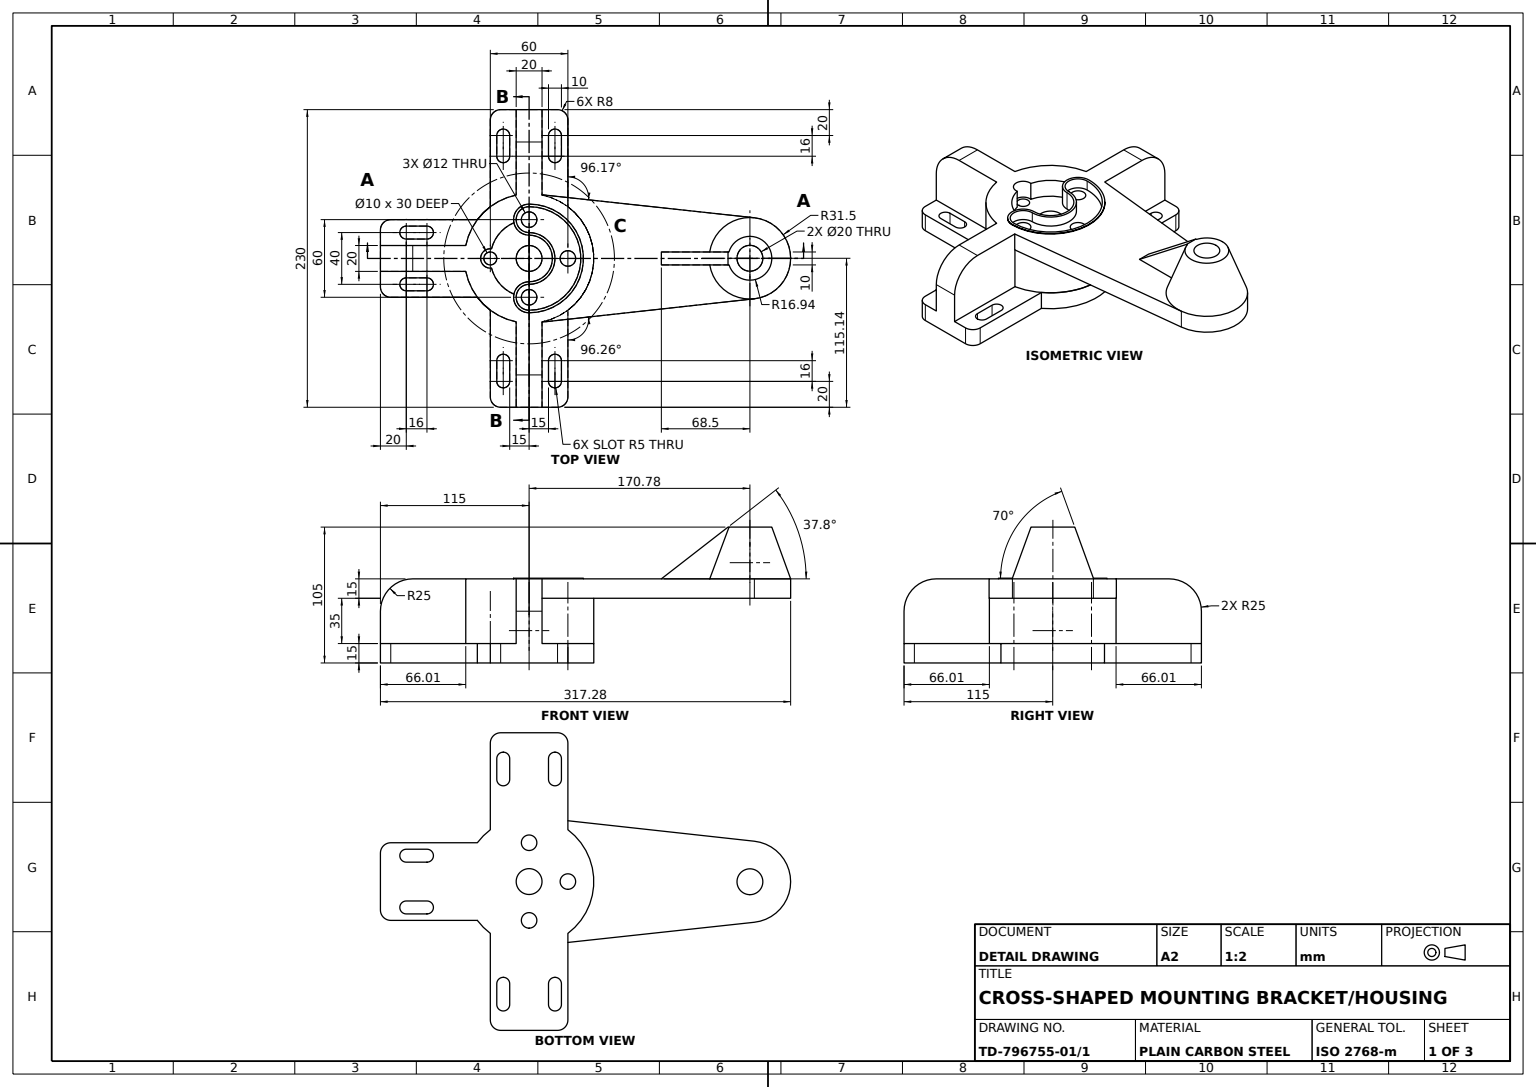
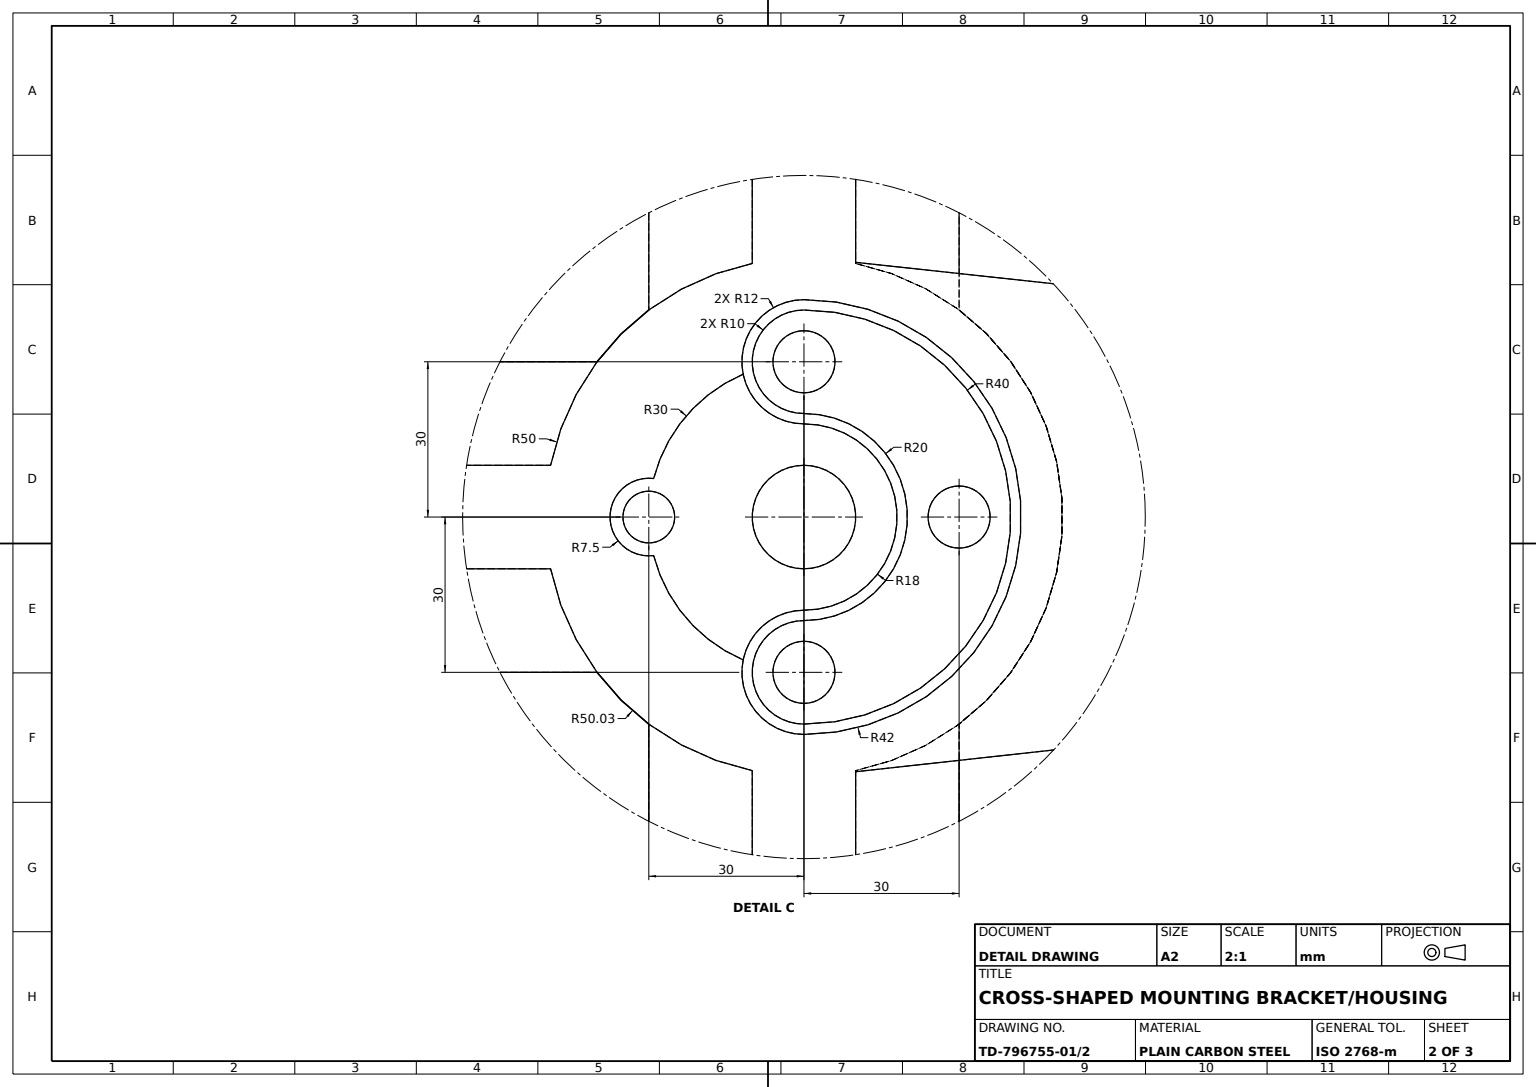
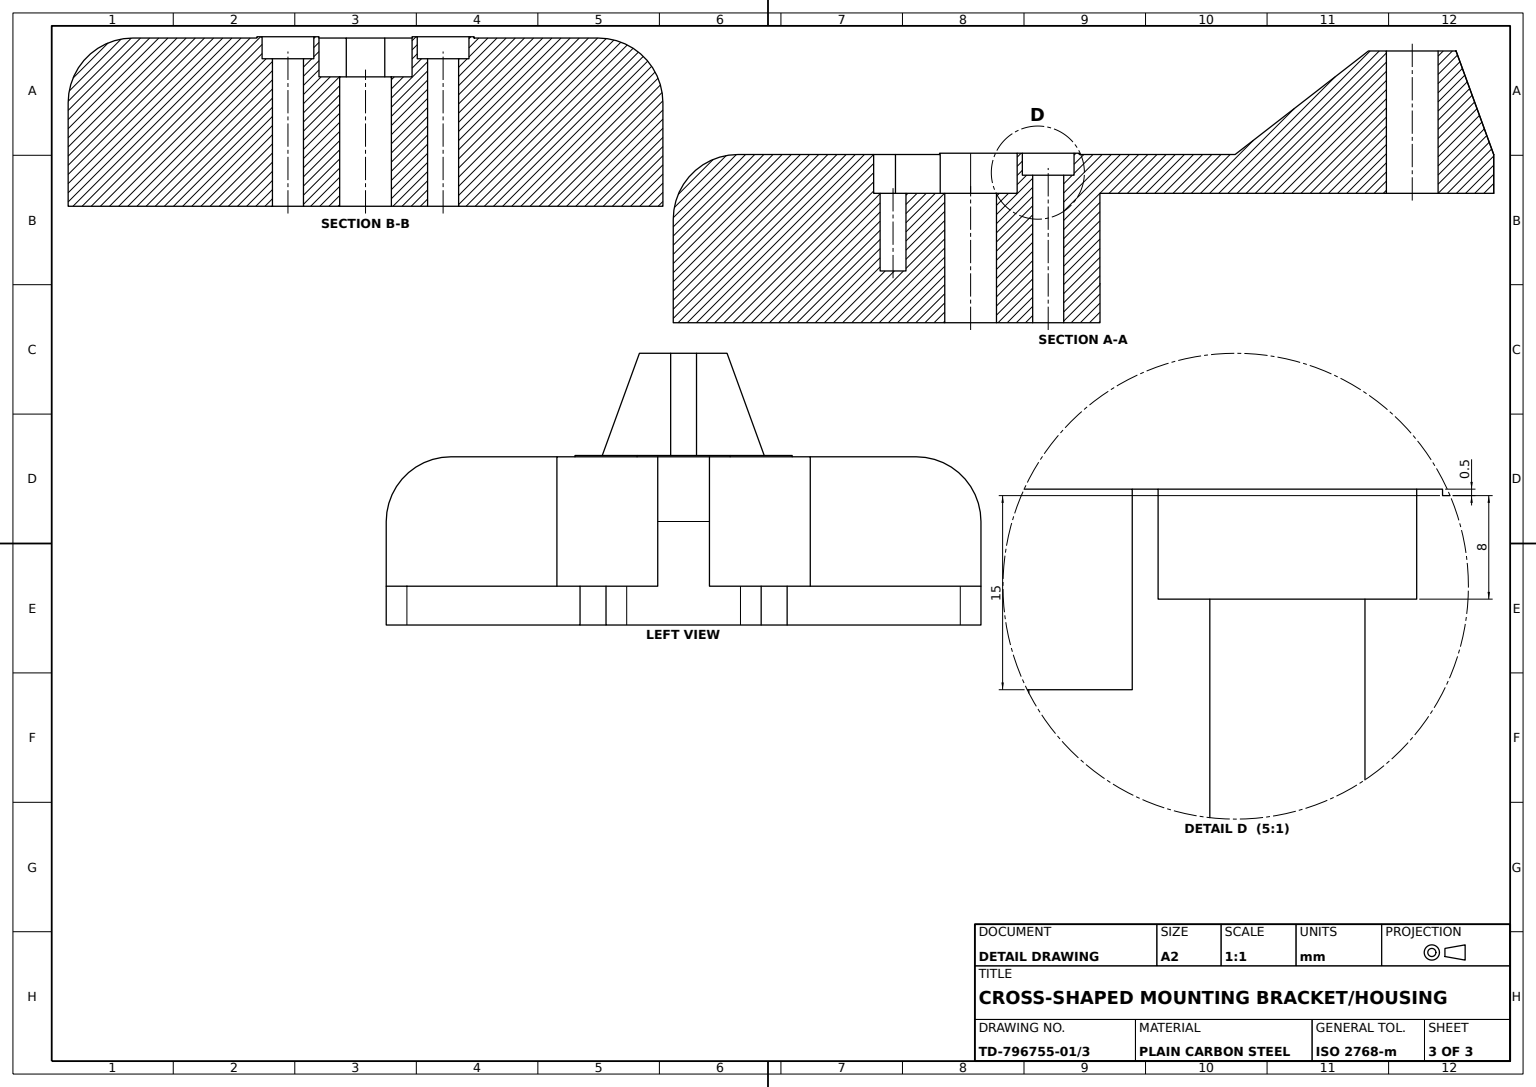
SolidWorks part; units mm, degrees
material "Plain Carbon Steel"
ref_plane "Front Plane" through (0, 0, 0) normal (0, 0, 1) x (1, 0, 0)
ref_plane "Top Plane" through (0, 0, 0) normal (0, 1, 0) x (1, 0, 0)
ref_plane "Right Plane" through (0, 0, 0) normal (1, 0, 0) x (0, 0, -1)
sketch "Cross Base Plate Sketch" plane through (0, 0, 0) normal (0, 1, 0) x (1, 0, 0)
  line L2 (30, 40.0427) -> (30, 107)
  line L3 (30, -107) -> (30, -40.0427)
  line L4 (-40.0427, 30) -> (-107, 30)
  line L5 (-30, -107) -> (-30, -40.0427)
  line L6 (-40.0427, -30) -> (-107, -30)
  line L7 (-115, 22) -> (-115, -22)
  line L8 (-22, 115) -> (22, 115)
  line L9 (-22, -115) -> (22, -115)
  line L10 (-30, 40.0427) -> (-30, 107)
  circle A0 centre (0, 0) radius 50.0341
  arc A1 (30, -107) -> (22, -115) centre (22, -107) cw
  arc A2 (-30, -107) -> (-22, -115) centre (-22, -107) ccw
  arc A3 (30, 107) -> (22, 115) centre (22, 107) ccw
  arc A4 (-30, 107) -> (-22, 115) centre (-22, 107) cw
  arc A5 (-107, -30) -> (-115, -22) centre (-107, -22) cw
  arc A6 (-107, 30) -> (-115, 22) centre (-107, 22) ccw
  point P3 (0, -115)
  point P4 (0, 115)
  point P6 (-115, 0)
  point P8 (0, 30)
  point P9 (-115, 30)
  point P10 (-30, -115)
  point P11 (-30, 115)
  dimension "D1" = 8
  dimension "D2" = 100.0683
  dimension "D3" = 74.9573
  dimension "D4" = 85
extrude "Cross Base Plate" add sketch "Cross Base Plate Sketch" along normal blind 15 contours L4 A6 L7 A5 L6 A0 | A0 | A4 L10 A0 L2 A3 L8 | L5 A2 L9 A1 L3 A0
sketch "Arm Slots Sketch" plane through (0, 15, 0) normal (0, 1, 0) x (1, 0, 0)
  line L0 (-95, 20) -> (-79, 20) construction
  line L1 (-115, 22) -> (-115, -22) construction
  line L2 (-95, 25) -> (-79, 25)
  line L3 (-95, 15) -> (-79, 15)
  line L4 (-40.0427, 30) -> (-107, 30) construction
  line L6 (-95, -20) -> (-79, -20) construction
  line L7 (-95, -25) -> (-79, -25)
  line L8 (-95, -15) -> (-79, -15)
  line L9 (-22, 115) -> (22, 115) construction
  line L11 (20, 95) -> (20, 79) construction
  line L12 (30, 40.0427) -> (30, 107) construction
  line L13 (25, 95) -> (25, 79)
  line L14 (15, 95) -> (15, 79)
  line L15 (-20, 95) -> (-20, 79) construction
  line L16 (-25, 95) -> (-25, 79)
  line L17 (-15, 95) -> (-15, 79)
  line L19 (20, -95) -> (20, -79) construction
  line L20 (25, -95) -> (25, -79)
  line L21 (15, -95) -> (15, -79)
  line L22 (-20, -95) -> (-20, -79) construction
  line L23 (-25, -95) -> (-25, -79)
  line L24 (-15, -95) -> (-15, -79)
  arc A0 (-95, 25) -> (-95, 15) centre (-95, 20) ccw
  arc A1 (-79, 15) -> (-79, 25) centre (-79, 20) ccw
  arc A2 (-95, -25) -> (-95, -15) centre (-95, -20) cw
  arc A3 (-79, -15) -> (-79, -25) centre (-79, -20) cw
  arc A4 (25, 95) -> (15, 95) centre (20, 95) ccw
  arc A5 (15, 79) -> (25, 79) centre (20, 79) ccw
  arc A6 (-25, 95) -> (-15, 95) centre (-20, 95) cw
  arc A7 (-15, 79) -> (-25, 79) centre (-20, 79) cw
  arc A9 (25, -95) -> (15, -95) centre (20, -95) cw
  arc A10 (15, -79) -> (25, -79) centre (20, -79) cw
  arc A11 (-25, -95) -> (-15, -95) centre (-20, -95) ccw
  arc A12 (-15, -79) -> (-25, -79) centre (-20, -79) ccw
  point P4 (-87, 20)
  point P16 (-87, -20)
  point P29 (20, 87)
  point P36 (-20, 87)
  point P48 (20, -87)
  point P55 (-20, -87)
  dimension "D1" = 5
  dimension "D2" = 16
  dimension "D5" = 5
  dimension "D9" = 5
  dimension "D10" = 5
  dimension "D11" = 95
  dimension "D12" = 50
  dimension "D13" = 109
  dimension "D14" = 117
  dimension "D3" = 20
  dimension "D4" = 5
  dimension "D6" = 16
  dimension "D7" = 20
  dimension "D8" = 5
extrude "Arm Slots" cut sketch "Arm Slots Sketch" against normal blind 15
sketch "Central Hub Sketch" plane through (0, 15, 0) normal (0, 1, 0) x (1, 0, 0)
  circle A0 centre (0, 0) radius 50
  dimension "D1" = 100
extrude "Central Hub Ø100" add sketch "Central Hub Sketch" along normal blind 50
sketch "Trunnion Arm Plate Sketch" plane through (0, 65, 0) normal (0, 1, 0) x (1, 0, 0)
  line L0 (5.3769, 49.7101) -> (174.172, 31.4524)
  line L1 (5.4555, -49.7015) -> (174.2216, -31.1768)
  arc A0 (174.2216, -31.1768) -> (174.172, 31.4524) centre (170.7846, 0.1351) ccw
  circle A3 centre (0, 0) radius 50
  circle A4 centre (0, 0) radius 50 construction
  circle M3 centre (0, 0) radius 50
  dimension "D1" = 63
  dimension "D2" = 100
  dimension "D3" = 5.3769
  dimension "D4" = 5.4555
  dimension "D5" = 170.7846
  dimension "D6" = 174.172
  dimension "D7" = 0.1351
extrude "Trunnion Arm Plate" add sketch "Trunnion Arm Plate Sketch" against normal blind 15 contours L1 A0 L0 M3
sketch "Trunnion Cone Sketch" plane through (0, 65, 0) normal (0, 1, 0) x (1, 0, 0)
  circle A0 centre (170.7846, 0.1351) radius 31.5
  dimension "D1" = 63
extrude "Trunnion Cone Boss" add sketch "Trunnion Cone Sketch" along normal blind 40 draft 20
sketch "Trunnion Bore Sketch" plane through (0, 105, 0) normal (0, 1, 0) x (1, 0, 0)
  circle A0 centre (170.7846, 0.1351) radius 10
  dimension "D1" = 20
extrude "Trunnion Bore Ø20" cut sketch "Trunnion Bore Sketch" against normal blind 100
ref_plane "Plane1" through (0, 0, 0) normal (0, 0, 1) x (1, 0, 0)
sketch "Trunnion Gusset Sketch" plane through (0, 0, 0) normal (0, 0, 1) x (1, 0, 0)
  line L0 (158.8434, 65) -> (102.2846, 65)
  line L1 (5.4555, 65) -> (174.2216, 65) construction
  line L2 (102.2846, 65) -> (153.8434, 105)
  line L3 (153.8434, 105) -> (158.8434, 105)
  line L4 (158.8434, 105) -> (158.8434, 65)
  dimension "D1" = 65.2557
  dimension "D2" = 56.5588
  dimension "D3" = 65
extrude "Trunnion Gusset" add sketch "Trunnion Gusset Sketch" along normal mid plane 10
ref_plane "Plane2" through (0, 0, 0) normal (0, 0, 1) x (1, 0, 0)
sketch "Arm Upright Block Sketch" plane through (0, 0, 0) normal (0, 0, 1) x (1, 0, 0)
  line L0 (-115, 15) -> (-115, 30)
  line L1 (-115, 30) -> (-115, 40)
  line L2 (-90, 65) -> (-42.4556, 65)
  line L3 (5.4555, 65) -> (-50, 65) construction
  line L4 (-42.4556, 65) -> (-42.4556, 15)
  line L5 (-40.0427, 15) -> (-107, 15) construction
  line L6 (-42.4556, 15) -> (-115, 15)
  arc A0 (-115, 40) -> (-90, 65) centre (-90, 40) cw
  dimension "D1" = 25
  dimension "D2" = 25
  dimension "D3" = 47.5444
  dimension "D4" = 15
extrude "Arm Upright Block" add sketch "Arm Upright Block Sketch" along normal mid plane 20
ref_plane "Plane3" through (0, 0, 0) normal (1, 0, 0) x (0, 0, -1)
sketch "Arm Upright Block Pair Sketch" plane through (0, 0, 0) normal (1, 0, 0) x (0, 0, -1)
  line L0 (115, 15) -> (115, 40)
  line L1 (90, 65) -> (40.208, 65)
  line L2 (50, 65) -> (10, 65) construction
  line L3 (40.208, 65) -> (40.0427, 15)
  line L4 (40.0427, 15) -> (115, 15)
  line L5 (-115, 15) -> (-115, 40)
  line L6 (-90, 65) -> (-41.4083, 65)
  line L7 (-10, 65) -> (-50, 65) construction
  line L8 (-41.4083, 65) -> (-41.4083, 15)
  line L9 (-107, 15) -> (-40.0427, 15) construction
  line L10 (-41.4083, 15) -> (-115, 15)
  arc A0 (115, 40) -> (90, 65) centre (90, 40) ccw
  arc A1 (-115, 40) -> (-90, 65) centre (-90, 40) cw
  dimension "D1" = 25
  dimension "D4" = 25
  dimension "D2" = 25
  dimension "D3" = 49.792
  dimension "D5" = 25
  dimension "D6" = 48.5917
extrude "Arm Upright Block Pair" add sketch "Arm Upright Block Pair Sketch" along normal mid plane 20
sketch "Central Bore Sketch" plane through (0, 65, 0) normal (0, 1, 0) x (1, 0, 0)
  circle A0 centre (0, 0) radius 10
  dimension "D1" = 20
extrude "Central Bore Ø20" cut sketch "Central Bore Sketch" against normal blind 200
sketch "Hub Top Recess Sketch" plane through (0, 65, 0) normal (0, 1, 0) x (1, 0, 0)
  arc A0 (-29.0625, -7.4412) -> (-29.0625, 7.4412) centre (0, 0) ccw
  arc A1 (-29.0625, 7.4412) -> (-29.0625, -7.4412) centre (-30, 0) ccw
  circle A2 centre (0, 0) radius 10
  dimension "D1" = 60
  dimension "D2" = 15
  dimension "D3" = 20
extrude "Hub Top Recess" cut sketch "Hub Top Recess Sketch" against normal blind 15
sketch "Hub Lobe Pocket Sketch" plane through (0, 65, 0) normal (0, 1, 0) x (1, 0, 0)
  arc A4 (0, 41) -> (0, 19) centre (0, 30) ccw
  arc A5 (0, -19) -> (0, -41) centre (0, -30) ccw
  arc A6 (0, 41) -> (0, -41) centre (0, 0) cw
  arc A7 (0, 19) -> (0, -19) centre (0, 0) cw
  dimension "D4" = 22
  dimension "D5" = 22
  dimension "D6" = 41
  dimension "D8" = 19
extrude "Hub Lobe Pocket" cut sketch "Hub Lobe Pocket Sketch" against normal blind 8
sketch "Pocket Floor Pad Sketch" plane through (0, 57, 0) normal (0, 1, 0) x (1, 0, 0)
  arc A0 (0, 41) -> (0, 19) centre (0, 30) ccw
  arc A1 (0, -19) -> (0, -41) centre (0, -30) ccw
  arc A2 (0, 19) -> (0, -19) centre (0, 0) cw
  arc A3 (0, 41) -> (0, -41) centre (0, 0) cw
  dimension "D2" = 22
  dimension "D3" = 41
  dimension "D4" = 19
extrude "Pocket Floor Pad" add sketch "Pocket Floor Pad Sketch" against normal blind 1
sketch "Pocket Thin Wall Sketch" plane through (0, 57, 0) normal (0, 1, 0) x (1, 0, 0)
  arc A0 (0, 41) -> (0, 19) centre (0, 30) ccw
  arc A1 (0, -19) -> (0, -41) centre (0, -30) ccw
  arc A2 (0, 19) -> (0, -19) centre (0, 0) cw
  arc A3 (0, 41) -> (0, -41) centre (0, 0) cw
  dimension "D1" = 41
  dimension "D2" = 19
extrude "Pocket Thin Wall" add sketch "Pocket Thin Wall Sketch" along normal blind 8.5 thin thin type one direction reverse wall 1
sketch "Hub Pin Holes Sketch" plane through (0, 57, 0) normal (0, 1, 0) x (1, 0, 0)
  circle A1 centre (0, 30) radius 6
  circle A2 centre (30, 0) radius 6
  circle A3 centre (0, -30) radius 6
  dimension "D1" = 12
  dimension "D2" = 12
  dimension "D3" = 12
  dimension "D4" = 30
  dimension "D5" = 10
  dimension "D6" = 40
  dimension "D7" = 70
extrude "Hub Pin Holes" cut sketch "Hub Pin Holes Sketch" against normal blind 200
sketch "Pocket Outer Wall Sketch" plane through (0, 65.5, 0) normal (0, 1, 0) x (1, 0, 0)
  arc A14 (0, -19) -> (0, -41) centre (0, -30) ccw
  arc A15 (0, -19) -> (0, 19) centre (0, 0) ccw
  arc A16 (0, -41) -> (0, 41) centre (0, 0) ccw
  arc A17 (0, 41) -> (0, 19) centre (0, 30) ccw
  arc A18 (0, -19) -> (0, -41) centre (0, -30) ccw
  arc A19 (0, -19) -> (0, 19) centre (0, 0) ccw
  arc A20 (0, -41) -> (0, 41) centre (0, 0) ccw
  arc A21 (0, 41) -> (0, 19) centre (0, 30) ccw
  dimension "D1" = 1
extrude "Pocket Outer Wall" add sketch "Pocket Outer Wall Sketch" against normal blind 50 thin
sketch "Pin Hole Bosses Sketch" plane through (0, 57, 0) normal (0, 1, 0) x (1, 0, 0)
  circle A15 centre (0, 30) radius 6
  circle A16 centre (30, 0) radius 6
  circle A17 centre (0, -30) radius 6
  arc A20 (-10.7778, -27.8) -> (0, -41) centre (0, -30) ccw
  arc A21 (0, -19) -> (-10.7778, -27.8) centre (0, -30) ccw
  arc A22 (0, -19) -> (0, 19) centre (0, 0) ccw
  arc A23 (0, -41) -> (0, 41) centre (0, 0) ccw
  arc A24 (0, 41) -> (0, 19) centre (0, 30) ccw
  arc A25 (-10.7778, -27.8) -> (0, -41) centre (0, -30) ccw
  arc A26 (0, -19) -> (-10.7778, -27.8) centre (0, -30) ccw
  arc A27 (0, -19) -> (0, 19) centre (0, 0) ccw
  arc A28 (0, -41) -> (0, 41) centre (0, 0) ccw
  arc A29 (0, 41) -> (0, 19) centre (0, 30) ccw
  dimension "D2" = 12
  dimension "D3" = 12
  dimension "D4" = 12
  dimension "D1" = 1
extrude "Pin Hole Bosses" add sketch "Pin Hole Bosses Sketch" against normal blind 20
sketch "Hub Side Hole Sketch" plane through (0, 50, 0) normal (0, 1, 0) x (1, 0, 0)
  circle A0 centre (-30, 0) radius 5
  dimension "D1" = 10
extrude "Hub Side Hole Ø10" cut sketch "Hub Side Hole Sketch" against normal blind 30
